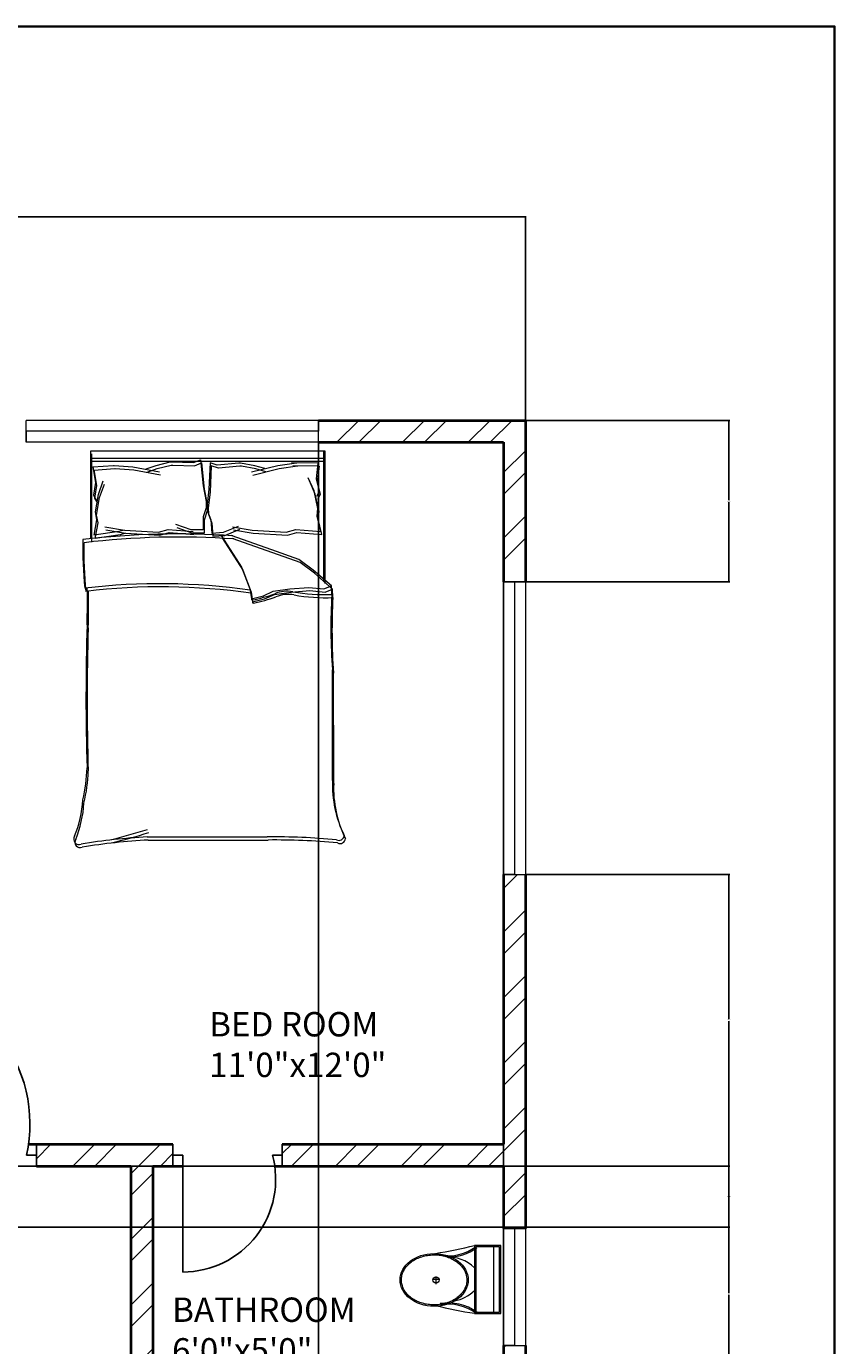
# Model space of a CAD drawing. Units: inches. Extents: x 2063 to 2617, y 1299 to 2210.
# Tile 22 of 22: x 2451 to 2617, y 1939 to 2210. Entities that reach past the tile are written whole.
import ezdxf

# ---------------------------------------------------------------- set-up
doc = ezdxf.new("R2010")
doc.units = ezdxf.units.IN
for name, color, linetype, lineweight in [('A-ANNO-DIMS', 2, 'Continuous', 18), ('A-ANNO-TTLB', 7, 'Continuous', 35), ('A-AREA-IDEN', 7, 'Continuous', 18), ('A-DOOR', 11, 'Continuous', 25), ('A-FLOR-FIXT', 8, 'Continuous', 18), ('A-FURN', 8, 'Continuous', 18), ('A-GLAZ', 123, 'Continuous', 18), ('A-WALL', 7, 'Continuous', 40)]:
    doc.layers.add(name, color=color, linetype=linetype, lineweight=lineweight)
doc.layers.add('A-WALL-PATT', color=215, linetype='Continuous', lineweight=13, true_color=0xa953a0)
doc.styles.get("Standard").update_dxf_attribs({"font": 'arial.ttf'})
doc.dimstyles.get("Standard").update_dxf_attribs({"dimtxt": 0.18, "dimasz": 0.18, "dimexe": 0.18, "dimexo": 0.0625, "dimgap": 0.09, "dimtad": 0, "dimtih": 1, "dimtoh": 1, "dimdec": 4, "dimzin": 0, "dimdsep": 46, "dimtxsty": 'Standard', "dimcen": 0.09, "dimadec": 0, "dimazin": 0, "dimtfac": 1, "dimtdec": 4, "dimtofl": 0, "dimtmove": 0, "dimatfit": 3, "dimfxl": 1, "dimtolj": 1, "dimtzin": 0, "dimarcsym": 0})

# ---------------------------------------------------------------- blocks, each defined once
blk = doc.blocks.new('A$C31115884')
for p, q in [((258, 466), (258, 523)), ((283, 498), (223, 498)), ((0, 200), (0, 0)), ((520, 200), (0, 200)), ((10, 190), (10, 10)), ((510, 190), (10, 190)), ((510, 10), (510, 190)), ((520, 0), (520, 200)), ((510, 54), (0, 54)), ((10, 10), (510, 10)), ((0, 0), (520, 0))]:
    blk.add_line(p, q)
blk.add_circle((256, 496), 23.6)
for centre, radius, start, end in [((2778, -205), 2807, 165.4549, 171.7133), ((-295, 403), 365, 324.2091, 9.3499), ((-295, 403), 375, 324.2091, 9.3499), ((139, 406), 293, 315.8436, 2.6563), ((806, 403), 375, 179.2036, 215.7909), ((806, 403), 365, 170.6501, 215.7909), ((3237, 905), 2807, 188.2867, 194.5451), ((384, 406), 293, 190.2774, 224.1564)]:
    blk.add_arc(centre, radius, start, end)
blk.add_ellipse((256, 510), major_axis=(0, -261), ratio=0.772727)
blk.add_open_spline([(256, 259), (263, 259), (270, 260), (288, 262), (299, 265), (320, 273), (330, 278), (350, 291), (360, 299), (378, 316), (386, 326), (402, 347), (409, 358), (421, 383), (427, 395), (436, 422), (440, 436), (445, 465), (447, 480), (448, 509), (448, 524), (445, 553), (443, 568), (436, 596), (432, 610), (422, 636), (416, 649), (402, 672), (395, 683), (379, 703), (370, 712), (351, 728), (341, 735), (321, 746), (310, 751), (289, 757), (278, 759), (256, 761), (245, 761), (223, 757), (212, 754), (191, 746), (181, 741), (161, 728), (151, 720), (133, 703), (125, 693), (110, 672), (103, 660), (90, 636), (85, 623), (76, 596), (72, 582), (67, 553), (66, 538), (64, 509), (65, 494), (68, 465), (70, 450), (77, 422), (81, 408), (91, 382), (97, 370), (111, 346), (118, 335), (135, 316), (144, 307), (162, 291), (172, 284), (193, 273), (203, 269), (225, 262), (236, 260), (250, 259), (253, 259), (256, 259)], degree=3, knots=[0, 0, 0, 0, 0.110105, 0.110105, 0.285049, 0.285049, 0.459994, 0.459994, 0.634938, 0.634938, 0.809882, 0.809882, 0.984827, 0.984827, 1.159771, 1.159771, 1.334715, 1.334715, 1.50966, 1.50966, 1.684604, 1.684604, 1.859549, 1.859549, 2.034493, 2.034493, 2.209437, 2.209437, 2.384382, 2.384382, 2.559326, 2.559326, 2.73427, 2.73427, 2.909215, 2.909215, 3.084159, 3.084159, 3.259103, 3.259103, 3.434048, 3.434048, 3.608992, 3.608992, 3.783936, 3.783936, 3.958881, 3.958881, 4.133825, 4.133825, 4.30877, 4.30877, 4.483714, 4.483714, 4.658658, 4.658658, 4.833603, 4.833603, 5.008547, 5.008547, 5.183491, 5.183491, 5.358436, 5.358436, 5.53338, 5.53338, 5.708324, 5.708324, 5.883269, 5.883269, 6.058213, 6.058213, 6.233158, 6.233158, 6.283185, 6.283185, 6.283185, 6.283185])
blk = doc.blocks.new('BED-DOUBLE')
for p, q in [((3.48, 63.33), (3.48, 81.44)), ((3.48, 63.33), (3.48, 81.44)), ((3.48, 81.44), (51.49, 81.44)), ((51.27, 81.44), (51.27, 54.83)), ((51.27, 81.44), (51.27, 54.83)), ((51.49, 81.44), (51.49, 80.8)), ((3.48, 79.91), (51.27, 79.91)), ((3.48, 79.91), (51.27, 79.91)), ((3.7, 62.69), (3.7, 80.8)), ((3.7, 62.69), (3.7, 80.8)), ((3.7, 79.27), (51.49, 79.27)), ((3.7, 79.27), (51.49, 79.27)), ((16.88, 78.42), (19.77, 79.14)), ((16.88, 78.42), (19.77, 79.14)), ((17.11, 77.78), (20, 78.5)), ((17.11, 77.78), (20, 78.5)), ((19.77, 79.14), (20.09, 79.14)), ((19.77, 79.14), (20.09, 79.14)), ((20, 78.5), (20.32, 78.5)), ((20, 78.5), (20.32, 78.5)), ((20.09, 79.14), (24.54, 79)), ((20.09, 79.14), (24.54, 79)), ((20.32, 78.5), (24.77, 78.36)), ((20.32, 78.5), (24.77, 78.36)), ((24.54, 79), (25.98, 79.57)), ((24.54, 79), (25.98, 79.57)), ((24.77, 78.36), (26.21, 78.93)), ((24.77, 78.36), (26.21, 78.93)), ((25.98, 79.57), (26.56, 74.22)), ((25.98, 79.57), (26.56, 74.22)), ((26.21, 78.93), (26.79, 73.58)), ((26.21, 78.93), (26.79, 73.58)), ((27.98, 78.95), (27.73, 73.58)), ((27.98, 78.95), (27.73, 73.58)), ((29.46, 78.46), (27.98, 78.95)), ((29.46, 78.46), (27.98, 78.95)), ((33.88, 78.89), (29.46, 78.46)), ((33.88, 78.89), (29.46, 78.46)), ((34.21, 78.91), (33.88, 78.89)), ((34.2, 78.91), (33.88, 78.89)), ((37.14, 78.37), (34.2, 78.91)), ((37.14, 78.37), (34.21, 78.91)), ((45.71, 78.9), (41.91, 78.37)), ((45.71, 78.9), (41.91, 78.37)), ((50.11, 78.89), (44.71, 78.98)), ((44.71, 78.98), (45.71, 78.9)), ((50.11, 78.89), (44.71, 78.98)), ((44.71, 78.98), (45.71, 78.9)), ((50.11, 78.89), (49.73, 75.68)), ((50.11, 78.89), (49.73, 75.68)), ((51.49, 80.8), (51.49, 54.19)), ((51.49, 80.8), (51.49, 54.19)), ((3.89, 78.13), (4.47, 74.95)), ((3.9, 78.11), (8.18, 78.43)), ((3.9, 78.11), (8.18, 78.43)), ((3.9, 78.13), (4.47, 74.95)), ((4.12, 77.49), (4.7, 74.31)), ((4.12, 77.49), (4.7, 74.31)), ((4.13, 77.47), (8.41, 77.8)), ((4.13, 77.47), (8.41, 77.8)), ((8.18, 78.43), (8.29, 78.42)), ((8.18, 78.43), (8.29, 78.42)), ((8.29, 78.42), (12.11, 78.13)), ((8.29, 78.42), (12.11, 78.13)), ((8.41, 77.8), (8.51, 77.78)), ((8.41, 77.8), (8.51, 77.78)), ((8.51, 77.78), (12.34, 77.49)), ((8.51, 77.78), (12.34, 77.49)), ((12.11, 78.13), (17.6, 77.12)), ((12.11, 78.13), (17.6, 77.12)), ((12.34, 77.49), (17.83, 76.48)), ((12.34, 77.49), (17.83, 76.48)), ((14.86, 77.69), (16.88, 78.42)), ((14.86, 77.69), (16.88, 78.42)), ((15.08, 77.05), (17.11, 77.78)), ((15.08, 77.05), (17.11, 77.78)), ((28.21, 78.31), (27.96, 72.94)), ((28.21, 78.31), (27.96, 72.94)), ((29.68, 77.83), (28.21, 78.31)), ((29.68, 77.83), (28.21, 78.31)), ((34.11, 78.25), (29.68, 77.83)), ((34.11, 78.25), (29.68, 77.83)), ((34.43, 78.27), (34.11, 78.25)), ((34.43, 78.27), (34.11, 78.25)), ((37.36, 77.73), (34.43, 78.27)), ((37.36, 77.73), (34.43, 78.27)), ((41.91, 78.37), (36.5, 77.02)), ((41.91, 78.37), (36.5, 77.02)), ((42.14, 77.73), (36.72, 76.38)), ((42.14, 77.73), (36.72, 76.38)), ((39.2, 77.77), (37.14, 78.37)), ((39.2, 77.77), (37.14, 78.37)), ((39.43, 77.13), (37.36, 77.73)), ((39.43, 77.13), (37.36, 77.73)), ((45.94, 78.26), (42.14, 77.73)), ((45.94, 78.26), (42.14, 77.73)), ((50.34, 78.25), (44.94, 78.34)), ((44.94, 78.34), (45.94, 78.26)), ((50.34, 78.25), (44.94, 78.34)), ((44.94, 78.34), (45.94, 78.26)), ((49.31, 73.19), (48.13, 75.87)), ((49.31, 73.19), (48.13, 75.87)), ((50.34, 78.25), (49.96, 75.04)), ((50.34, 78.25), (49.96, 75.04)), ((4.47, 74.95), (4.04, 72.34)), ((4.47, 74.95), (4.04, 72.34)), ((4.7, 74.31), (4.27, 71.7)), ((4.7, 74.31), (4.27, 71.7)), ((5.05, 72.49), (6.06, 75.24)), ((5.05, 72.49), (6.06, 75.24)), ((5.28, 71.85), (6.29, 74.6)), ((5.28, 71.85), (6.29, 74.6)), ((26.56, 74.22), (27.14, 71.04)), ((26.56, 74.22), (27.14, 71.04)), ((26.79, 73.58), (27.37, 70.4)), ((26.79, 73.58), (27.37, 70.4)), ((27.73, 73.58), (27.36, 70.37)), ((27.73, 73.58), (27.36, 70.37)), ((49.54, 72.55), (48.36, 75.23)), ((49.54, 72.55), (48.36, 75.23)), ((50.11, 69.61), (49.31, 73.19)), ((50.11, 69.61), (49.31, 73.19)), ((49.73, 75.68), (50.33, 73.11)), ((49.73, 75.68), (50.33, 73.11)), ((50.33, 73.11), (49.81, 72.06)), ((50.33, 73.11), (49.82, 72.06)), ((49.96, 75.04), (50.56, 72.47)), ((49.96, 75.04), (50.56, 72.47)), ((4.04, 72.34), (4.62, 71.33)), ((4.04, 72.34), (4.62, 71.33)), ((4.27, 71.7), (4.85, 70.69)), ((4.27, 71.7), (4.85, 70.69)), ((4.47, 68.87), (5.05, 72.49)), ((4.47, 68.87), (5.05, 72.49)), ((4.7, 68.23), (5.28, 71.85)), ((4.7, 68.23), (5.28, 71.85)), ((27.14, 71.04), (27.14, 69.74)), ((27.14, 71.04), (27.14, 69.74)), ((27.37, 70.4), (27.37, 69.1)), ((27.37, 70.4), (27.37, 69.1)), ((27.96, 72.94), (27.58, 69.73)), ((27.96, 72.94), (27.58, 69.73)), ((50.34, 68.98), (49.54, 72.55)), ((50.34, 68.98), (49.54, 72.55)), ((50.56, 72.47), (50.04, 71.42)), ((50.56, 72.47), (50.04, 71.42)), ((4.76, 67.28), (4.47, 68.87)), ((4.76, 67.28), (4.47, 68.87)), ((4.99, 66.64), (4.7, 68.23)), ((4.99, 66.64), (4.7, 68.23)), ((27.14, 69.74), (26.56, 67.86)), ((27.14, 69.74), (26.56, 67.86)), ((26.56, 67.86), (26.56, 65.18)), ((26.56, 67.86), (26.56, 65.18)), ((27.37, 69.1), (26.79, 67.22)), ((27.37, 69.1), (26.79, 67.22)), ((27.36, 70.37), (27.44, 69.07)), ((27.36, 70.37), (27.44, 69.07)), ((27.44, 69.07), (28.13, 67.23)), ((27.44, 69.07), (28.13, 67.23)), ((27.58, 69.73), (27.66, 68.43)), ((27.58, 69.73), (27.66, 68.43)), ((27.66, 68.43), (28.36, 66.59)), ((27.66, 68.43), (28.36, 66.59)), ((49.92, 68.01), (50.11, 69.61)), ((49.92, 68.01), (50.11, 69.61)), ((50.7, 64.87), (49.92, 68.01)), ((50.7, 64.87), (49.92, 68.01)), ((50.15, 67.37), (50.34, 68.98)), ((50.15, 67.37), (50.34, 68.98)), ((4.18, 64.1), (4.76, 67.28)), ((4.18, 64.1), (4.76, 67.28)), ((4.41, 63.46), (4.99, 66.64)), ((4.41, 63.46), (4.99, 66.64)), ((6.38, 65.82), (10.41, 65.15)), ((6.38, 65.82), (10.41, 65.15)), ((6.61, 65.18), (10.64, 64.51)), ((6.61, 65.18), (10.64, 64.51)), ((10.41, 65.15), (9.28, 64.83)), ((10.41, 65.15), (9.28, 64.83)), ((10.41, 65.15), (17.42, 64.72)), ((10.41, 65.15), (17.42, 64.72)), ((17.42, 64.72), (19.38, 65.27)), ((17.42, 64.72), (19.38, 65.27)), ((19.38, 65.27), (24.52, 64.87)), ((19.38, 65.27), (24.52, 64.87)), ((24.1, 65.18), (20.96, 66.27)), ((24.1, 65.18), (20.96, 66.27)), ((24.33, 64.54), (21.19, 65.63)), ((24.33, 64.54), (21.19, 65.63)), ((26.56, 65.18), (24.1, 65.18)), ((26.56, 65.18), (24.1, 65.18)), ((26.79, 67.22), (26.79, 64.54)), ((26.79, 67.22), (26.79, 64.54)), ((28.13, 67.23), (28.3, 64.55)), ((28.13, 67.23), (28.3, 64.55)), ((28.36, 66.59), (28.53, 63.91)), ((28.36, 66.59), (28.53, 63.91)), ((30.75, 64.7), (33.82, 65.99)), ((30.75, 64.7), (33.82, 65.99)), ((30.98, 64.06), (34.05, 65.35)), ((30.98, 64.06), (34.05, 65.35)), ((32.56, 65.82), (36.6, 65.15)), ((32.56, 65.82), (36.6, 65.15)), ((32.79, 65.18), (36.83, 64.51)), ((32.79, 65.18), (36.82, 64.51)), ((36.6, 65.15), (43.61, 64.72)), ((36.6, 65.15), (43.61, 64.72)), ((43.61, 64.72), (45.57, 65.27)), ((43.61, 64.72), (45.57, 65.27)), ((45.57, 65.27), (50.7, 64.87)), ((45.57, 65.27), (50.7, 64.87)), ((50.93, 64.23), (50.15, 67.37)), ((50.93, 64.23), (50.15, 67.37)), ((9.28, 64.83), (4.18, 64.1)), ((9.28, 64.83), (4.18, 64.1)), ((9.51, 64.19), (4.41, 63.46)), ((9.51, 64.19), (4.41, 63.46)), ((10.64, 64.51), (9.51, 64.19)), ((10.64, 64.51), (9.51, 64.19)), ((10.64, 64.51), (17.65, 64.08)), ((10.64, 64.51), (17.65, 64.08)), ((17.65, 64.08), (19.61, 64.64)), ((17.65, 64.08), (19.61, 64.64)), ((19.61, 64.64), (24.74, 64.23)), ((19.61, 64.64), (24.74, 64.23)), ((26.79, 64.54), (24.33, 64.54)), ((26.79, 64.54), (24.33, 64.54)), ((28.3, 64.55), (30.75, 64.7)), ((28.3, 64.55), (30.75, 64.7)), ((28.53, 63.91), (30.98, 64.06)), ((28.53, 63.91), (30.98, 64.06)), ((30.26, 64.06), (34.45, 57.57)), ((30.26, 64.06), (34.45, 57.57)), ((30.49, 63.42), (34.68, 56.93)), ((30.49, 63.42), (34.68, 56.93)), ((40.64, 61.13), (32.31, 64.06)), ((40.64, 61.13), (32.31, 64.06)), ((40.87, 60.49), (32.53, 63.42)), ((40.87, 60.49), (32.54, 63.42)), ((36.82, 64.51), (43.83, 64.08)), ((36.83, 64.51), (43.84, 64.08)), ((43.83, 64.08), (45.8, 64.64)), ((43.84, 64.08), (45.8, 64.64)), ((45.8, 64.64), (50.93, 64.23)), ((45.8, 64.64), (50.93, 64.23)), ((46.22, 59.11), (40.64, 61.13)), ((46.22, 59.11), (40.64, 61.13)), ((46.45, 58.48), (40.87, 60.49)), ((46.45, 58.48), (40.87, 60.49)), ((34.45, 57.57), (36.15, 53.08)), ((34.45, 57.57), (36.15, 53.08)), ((34.68, 56.93), (36.38, 52.44)), ((34.68, 56.93), (36.38, 52.44)), ((49.16, 56.95), (46.22, 59.11)), ((49.16, 56.95), (46.22, 59.11)), ((49.39, 56.31), (46.45, 58.48)), ((49.39, 56.31), (46.45, 58.48)), ((52.87, 53.7), (49.16, 56.95)), ((52.87, 53.7), (49.16, 56.95)), ((53.1, 53.06), (49.39, 56.31)), ((53.1, 53.06), (49.39, 56.31)), ((36.15, 53.08), (36.46, 51.07)), ((36.15, 53.08), (36.46, 51.07)), ((36.38, 52.44), (36.69, 50.43)), ((36.38, 52.44), (36.69, 50.43)), ((36.46, 51.07), (38.94, 51.69)), ((36.46, 51.07), (38.94, 51.69)), ((38.94, 51.69), (40.95, 52.61)), ((38.94, 51.69), (40.95, 52.61)), ((39.17, 51.05), (41.18, 51.97)), ((39.17, 51.05), (41.18, 51.97)), ((40.95, 52.61), (44.36, 53.08)), ((40.95, 52.61), (44.36, 53.08)), ((41.18, 51.97), (44.59, 52.44)), ((41.18, 51.97), (44.59, 52.44)), ((44.36, 53.08), (48.23, 53.39)), ((44.36, 53.08), (48.23, 53.39)), ((44.59, 52.44), (48.46, 52.75)), ((44.59, 52.44), (48.46, 52.75)), ((48.23, 53.39), (51.33, 53.08)), ((48.23, 53.39), (51.33, 53.08)), ((48.46, 52.75), (51.56, 52.44)), ((48.46, 52.75), (51.56, 52.44)), ((51.33, 53.08), (52.87, 53.7)), ((51.33, 53.08), (52.87, 53.7)), ((51.56, 52.44), (53.1, 53.06)), ((51.56, 52.44), (53.1, 53.06)), ((52.95, 51.95), (52.87, 53.7, 3.87)), ((52.95, 51.95), (52.87, 53.7, 3.87)), ((53.18, 51.31), (53.1, 53.06, 3.87)), ((53.18, 51.31), (53.1, 53.06, 3.87)), ((36.69, 50.43), (39.17, 51.05)), ((36.69, 50.43), (39.17, 51.05)), ((15.06, 2.2), (39.68, 2.2)), ((15.06, 2.2), (39.68, 2.2)), ((15.29, 1.56), (39.91, 1.56)), ((15.29, 1.56), (39.91, 1.56))]:
    blk.add_line(p, q)
for centre, radius, start, end in [((85.16, 61.35), 83.31, 178.7218, 185.604), ((85.16, 61.35), 83.31, 178.7218, 185.604), ((21.36, -100.61), 164.97, 86.0865, 96.7821), ((21.36, -100.61), 164.97, 86.0865, 96.7821), ((85.39, 60.71), 83.31, 178.7218, 185.604), ((85.39, 60.71), 83.31, 178.7218, 185.604), ((21.59, -101.25), 164.97, 86.0865, 96.7821), ((21.59, -101.25), 164.97, 86.0865, 96.7821), ((17.76, -74.87), 129.02, 81.7845, 96.9006), ((17.76, -74.87), 129.02, 81.7845, 96.9006), ((17.98, -75.51), 129.02, 81.7845, 96.9006), ((17.98, -75.51), 129.02, 81.7845, 96.9006), ((-167.31, 50.27), 170.11, 358.4762, 1.0082), ((-167.31, 50.27), 170.11, 358.4762, 1.0082), ((-167.08, 49.63), 170.11, 358.4762, 1.0082), ((-167.08, 49.63), 170.11, 358.4762, 1.0082), ((31.15, 79.96), 29.65, 280.6617, 289.8806), ((31.15, 79.96), 29.65, 280.6617, 289.8806), ((31.38, 79.32), 29.65, 280.6617, 289.8806), ((31.38, 79.32), 29.65, 280.6617, 289.8806), ((43.74, 46.38), 6.22, 78.6608, 113.7384), ((43.74, 46.38), 6.22, 78.6608, 113.7384), ((43.97, 45.74), 6.22, 78.6608, 113.7384), ((43.97, 45.74), 6.22, 78.6608, 113.7384), ((51.33, 88.1), 36.18, 259.8763, 272.5657), ((51.33, 88.1), 36.18, 259.8763, 272.5657), ((51.56, 87.46), 36.18, 259.8763, 272.5657), ((51.56, 87.46), 36.18, 259.8763, 272.5657), ((182.27, 45.13), 129.5, 176.9791, 183.8365), ((182.27, 45.13), 129.5, 176.9791, 183.8365), ((36.64, 51), 0.185, 160.2464, 271.1377), ((36.64, 51), 0.185, 160.2464, 271.1377), ((36.87, 50.36), 0.185, 160.2464, 271.1377), ((36.86, 50.36), 0.185, 160.2464, 271.1377), ((182.49, 44.49), 129.5, 176.9791, 183.8365), ((182.49, 44.49), 129.5, 176.9791, 183.8365), ((484.82, 30.83), 482.31, 178.2277, 181.7185), ((484.82, 30.83), 482.31, 178.2277, 181.7185), ((485.05, 30.19), 482.31, 178.2277, 181.7185), ((485.05, 30.19), 482.31, 178.2277, 181.7185), ((-4508.74, 13.62), 4561.86, 0.00217, 0.28689), ((-4508.74, 13.62), 4561.86, 0.00217, 0.28689), ((-4508.51, 12.98), 4561.86, 0.00217, 0.28689), ((-4508.51, 12.98), 4561.86, 0.00217, 0.28689), ((-26.9, 16.93), 29.63, 346.0648, 358.9113), ((-26.9, 16.93), 29.63, 346.0648, 358.9113), ((-26.67, 16.29), 29.63, 346.0648, 358.9113), ((-26.67, 16.29), 29.63, 346.0648, 358.9113), ((76.16, 12.78), 23.07, 177.4714, 206.4681), ((76.16, 12.78), 23.07, 177.4714, 206.4681), ((76.39, 12.14), 23.07, 177.4714, 206.4681), ((76.39, 12.14), 23.07, 177.4714, 206.4681), ((-21.66, 11.17), 23.56, 337.9751, 356.652), ((-21.66, 11.17), 23.56, 337.9751, 356.652), ((-21.43, 10.53), 23.56, 337.9751, 356.652), ((-21.43, 10.53), 23.56, 337.9751, 356.652), ((-17.22, 105.16), 106.46, 283.3832, 287.7053), ((-17.22, 105.16), 106.46, 283.3832, 287.7053), ((-16.99, 104.52), 106.46, 283.3832, 287.7053), ((-16.99, 104.52), 106.46, 283.3832, 287.7053), ((1.09, 1.73), 1.09, 146.1736, 293.4781), ((1.09, 1.73), 1.09, 146.1736, 293.4781), ((1.32, 1.09), 1.09, 146.1736, 293.4781), ((1.32, 1.09), 1.09, 146.1736, 293.4781), ((21.43, -119.39), 121.76, 92.9958, 99.4091), ((21.43, -119.39), 121.76, 92.9958, 99.4091), ((21.66, -120.03), 121.76, 92.9958, 99.4091), ((21.66, -120.03), 121.76, 92.9958, 99.4091), ((41.15, -130.83), 133.04, 84.4998, 90.6351), ((41.15, -130.83), 133.04, 84.4998, 90.6351), ((41.38, -131.47), 133.04, 84.4998, 90.6351), ((41.38, -131.47), 133.04, 84.4998, 90.6351), ((54.41, 2.57), 1.1, 242.6588, 356.02), ((54.41, 2.57), 1.1, 242.6588, 356.02), ((54.64, 1.93), 1.1, 242.6588, 356.02), ((54.64, 1.93), 1.1, 242.6588, 356.02)]:
    blk.add_arc(centre, radius, start, end)
blk = doc.blocks.new('WIN-60IN')
for p, q in [((0, 60), (4.5, 60)), ((0, 60), (0, 0)), ((4.5, 60), (2.25, 60)), ((2.25, 60), (2.25, 0)), ((4.5, 60), (4.5, 0)), ((2.25, 0), (0, 0)), ((0, 0), (4.5, 0))]:
    blk.add_line(p, q)
blk = doc.blocks.new('WIN-24IN')
for p, q in [((0, 24), (4.5, 24)), ((0, 24), (0, 0)), ((4.5, 24), (2.25, 24)), ((2.25, 24), (2.25, 0)), ((4.5, 24), (4.5, 0)), ((2.25, 0), (0, 0)), ((0, 0), (4.5, 0))]:
    blk.add_line(p, q)
blk = doc.blocks.new('*D31')
at = {"layer": 'A-ANNO-DIMS', "color": 0, "lineweight": -2, "transparency": 16777216}
for p, q in [((2123.14, 2128.87), (2123.14, 2170.74)), ((2123.32, 2170.56), (2338, 2170.56)), ((2553.46, 2170.56), (2338.79, 2170.56)), ((2553.64, 2128.87), (2553.64, 2170.74))]:
    blk.add_line(p, q, dxfattribs=at)
at = {"layer": 'A-ANNO-DIMS', "color": 0, "transparency": 16777216}
for points in [[(2123.32, 2170.59), (2123.32, 2170.53), (2123.14, 2170.56)], [(2553.46, 2170.59), (2553.46, 2170.53), (2553.64, 2170.56)]]:
    blk.add_solid(points, dxfattribs=at)
at = {"layer": 'Defpoints', "color": 0, "transparency": 16777216}
for p in [(2553.64, 2170.56), (2123.14, 2128.81), (2553.64, 2128.81)]:
    blk.add_point(p, dxfattribs=at)
at = {"layer": 'A-ANNO-DIMS', "color": 0, "transparency": 16777216, "insert": (2338.39, 2170.56), "char_height": 0.18, "attachment_point": 5}
blk.add_mtext('\\A1;430.5', dxfattribs=at)
blk = doc.blocks.new('*D46')
at = {"layer": 'A-ANNO-DIMS', "color": 0, "lineweight": -2, "transparency": 16777216}
for p, q in [((2549.21, 1975.81), (2595.57, 1975.81)), ((2595.39, 1975.63), (2595.39, 1949.74)), ((2595.39, 1923.49), (2595.39, 1949.38)), ((2549.21, 1923.31), (2595.57, 1923.31))]:
    blk.add_line(p, q, dxfattribs=at)
at = {"layer": 'A-ANNO-DIMS', "color": 0, "transparency": 16777216}
for points in [[(2595.36, 1975.63), (2595.42, 1975.63), (2595.39, 1975.81)], [(2595.36, 1923.49), (2595.42, 1923.49), (2595.39, 1923.31)]]:
    blk.add_solid(points, dxfattribs=at)
at = {"layer": 'Defpoints', "color": 0, "transparency": 16777216}
for p in [(2549.14, 1975.81), (2595.39, 1975.81), (2549.14, 1923.31)]:
    blk.add_point(p, dxfattribs=at)
at = {"layer": 'A-ANNO-DIMS', "color": 0, "transparency": 16777216, "insert": (2595.39, 1949.56), "char_height": 0.18, "attachment_point": 5}
blk.add_mtext('\\A1;52.5', dxfattribs=at)
blk = doc.blocks.new('*D47')
at = {"layer": 'A-ANNO-DIMS', "color": 0, "lineweight": -2, "transparency": 16777216}
for p, q in [((2553.71, 2035.66), (2595.57, 2035.66)), ((2595.39, 2035.48), (2595.39, 2005.92)), ((2595.39, 1975.99), (2595.39, 2005.56)), ((2549.21, 1975.81), (2595.57, 1975.81))]:
    blk.add_line(p, q, dxfattribs=at)
at = {"layer": 'A-ANNO-DIMS', "color": 0, "transparency": 16777216}
for points in [[(2595.36, 2035.48), (2595.42, 2035.48), (2595.39, 2035.66)], [(2595.36, 1975.99), (2595.42, 1975.99), (2595.39, 1975.81)]]:
    blk.add_solid(points, dxfattribs=at)
at = {"layer": 'Defpoints', "color": 0, "transparency": 16777216}
for p in [(2553.64, 2035.66), (2595.39, 2035.66), (2549.14, 1975.81)]:
    blk.add_point(p, dxfattribs=at)
at = {"layer": 'A-ANNO-DIMS', "color": 0, "transparency": 16777216, "insert": (2595.39, 2005.74), "char_height": 0.18, "attachment_point": 5}
blk.add_mtext('\\A1;59.85', dxfattribs=at)
blk = doc.blocks.new('*D48')
at = {"layer": 'A-ANNO-DIMS', "color": 0, "lineweight": -2, "transparency": 16777216}
for p, q in [((2553.71, 2128.81), (2595.57, 2128.81)), ((2595.39, 2128.63), (2595.39, 2112.42)), ((2595.39, 2095.84), (2595.39, 2112.06)), ((2549.21, 2095.66), (2595.57, 2095.66))]:
    blk.add_line(p, q, dxfattribs=at)
at = {"layer": 'A-ANNO-DIMS', "color": 0, "transparency": 16777216}
for points in [[(2595.36, 2128.63), (2595.42, 2128.63), (2595.39, 2128.81)], [(2595.36, 2095.84), (2595.42, 2095.84), (2595.39, 2095.66)]]:
    blk.add_solid(points, dxfattribs=at)
at = {"layer": 'Defpoints', "color": 0, "transparency": 16777216}
for p in [(2553.64, 2128.81), (2595.39, 2128.81), (2549.14, 2095.66)]:
    blk.add_point(p, dxfattribs=at)
at = {"layer": 'A-ANNO-DIMS', "color": 0, "transparency": 16777216, "insert": (2595.39, 2112.24), "char_height": 0.18, "attachment_point": 5}
blk.add_mtext('\\A1;33.15', dxfattribs=at)
blk = doc.blocks.new('*D52')
at = {"layer": 'A-ANNO-DIMS', "color": 0, "lineweight": -2, "transparency": 16777216}
for p, q in [((2511.17, 2124.25), (2511.17, 1317.7)), ((2549.14, 2124.25), (2549.14, 1317.7)), ((2511.35, 1317.88), (2529.69, 1317.88)), ((2548.96, 1317.88), (2530.62, 1317.88))]:
    blk.add_line(p, q, dxfattribs=at)
at = {"layer": 'A-ANNO-DIMS', "color": 0, "transparency": 16777216}
for points in [[(2511.35, 1317.91), (2511.35, 1317.85), (2511.17, 1317.88)], [(2548.96, 1317.91), (2548.96, 1317.85), (2549.14, 1317.88)]]:
    blk.add_solid(points, dxfattribs=at)
at = {"layer": 'Defpoints', "color": 0, "transparency": 16777216}
for p in [(2511.17, 2124.31), (2549.14, 2124.31), (2549.14, 1317.88)]:
    blk.add_point(p, dxfattribs=at)
at = {"layer": 'A-ANNO-DIMS', "color": 0, "transparency": 16777216, "insert": (2530.16, 1317.88), "char_height": 0.18, "attachment_point": 5}
blk.add_mtext('\\A1;37.974', dxfattribs=at)
blk = doc.blocks.new('*D67')
at = {"layer": 'A-ANNO-DIMS', "color": 0, "lineweight": -2, "transparency": 16777216}
for p, q in [((2127.71, 1975.81), (2595.57, 1975.81)), ((2595.39, 1975.63), (2595.39, 1969.73)), ((2595.39, 1963.46), (2595.39, 1969.36)), ((2128.42, 1963.28), (2595.57, 1963.28))]:
    blk.add_line(p, q, dxfattribs=at)
at = {"layer": 'A-ANNO-DIMS', "color": 0, "transparency": 16777216}
for points in [[(2595.36, 1975.63), (2595.42, 1975.63), (2595.39, 1975.81)], [(2595.36, 1963.46), (2595.42, 1963.46), (2595.39, 1963.28)]]:
    blk.add_solid(points, dxfattribs=at)
at = {"layer": 'Defpoints', "color": 0, "transparency": 16777216}
for p in [(2127.64, 1975.81), (2128.36, 1963.28), (2595.39, 1963.28)]:
    blk.add_point(p, dxfattribs=at)
at = {"layer": 'A-ANNO-DIMS', "color": 0, "transparency": 16777216, "insert": (2595.39, 1969.55), "char_height": 0.18, "attachment_point": 5}
blk.add_mtext('\\A1;12.533', dxfattribs=at)

msp = doc.modelspace()

# ---------------------------------------------------------------- hatches: boundary and pattern name
at = {"layer": 'A-WALL-PATT'}
h = msp.add_hatch(dxfattribs=at)
h.set_pattern_fill('ANSI32', color=256)
h.paths.add_polyline_path([(2553.6442, 2128.8122), (2511.1703, 2128.8122), (2511.1703, 2124.3122), (2549.1442, 2124.3122), (2549.1442, 2095.662), (2553.6442, 2095.662)])
h.paths.add_polyline_path([(2553.6442, 2035.662), (2549.1442, 2035.662), (2549.1442, 1980.3122), (2503.7214, 1980.3122), (2503.7214, 1975.8122), (2549.1442, 1975.8122), (2549.1442, 1962.9693), (2553.6442, 1962.9693)])
h.paths.add_polyline_path([(2553.6442, 1938.9693), (2549.1442, 1938.9693), (2549.1442, 1927.8122), (2477.1442, 1927.8122), (2477.1442, 1975.8122), (2481.2918, 1975.8122), (2481.2918, 1980.3122), (2453.2648, 1980.3122), (2453.2648, 1975.8122), (2472.6442, 1975.8122), (2472.6442, 1868.3122), (2400.6442, 1868.3122), (2400.6442, 1861.3782), (2405.1442, 1861.3782), (2405.1442, 1863.8122), (2480.9699, 1863.8122), (2480.9699, 1866.0622), (2480.9699, 1868.3122), (2477.1442, 1868.3122), (2477.1442, 1923.3122), (2549.1442, 1923.3122), (2549.1442, 1908.8504), (2553.6442, 1908.8504)])
h.paths.add_polyline_path([(2553.6442, 1884.8504), (2549.1442, 1884.8504), (2549.1442, 1868.3122), (2501.0636, 1868.3122), (2501.0636, 1863.8122), (2549.1442, 1863.8122), (2549.1442, 1826.0298), (2553.6442, 1826.0298)])
h.paths.add_polyline_path([(2388.1504, 1980.3122), (2340.6442, 1980.3122), (2340.6442, 2124.3122), (2358.7501, 2124.3122), (2358.7501, 2128.8122), (2316.3482, 2128.8122), (2316.3482, 2124.3122), (2336.1442, 2124.3122), (2336.1442, 1980.3122), (2289.1737, 1980.3122), (2289.1737, 1975.8122), (2336.1442, 1975.8122), (2336.1442, 1619.3122), (2333.1433, 1619.3122), (2333.1433, 1614.8122), (2344.1671, 1614.8122), (2344.1671, 1617.0622), (2344.1671, 1619.3122), (2340.6442, 1619.3122), (2340.6442, 1975.8122), (2388.1504, 1975.8122), (2388.1504, 1978.0622)])
h.paths.add_polyline_path([(2290.1442, 1614.8122), (2301.4594, 1614.8122), (2301.4594, 1617.0622), (2301.4594, 1619.3122), (2285.6442, 1619.3122), (2285.6442, 1566.8122), (2280.8619, 1566.8122), (2280.8619, 1564.5622), (2280.8619, 1562.3122), (2285.6442, 1562.3122), (2285.6442, 1442.3122), (2281.7879, 1442.3122), (2281.7879, 1437.8122), (2285.6442, 1437.8122), (2285.6442, 1401.8122), (2290.1442, 1401.8122)])
h.paths.add_polyline_path([(2549.1442, 1731.8122), (2405.1442, 1731.8122), (2405.1442, 1834.4638), (2402.8942, 1834.4638), (2400.6442, 1834.4638), (2400.6442, 1727.3122), (2549.1442, 1727.3122)])
h.paths.add_polyline_path([(2553.6442, 1766.0298), (2551.3942, 1766.0298), (2549.1442, 1766.0298), (2549.1442, 1686.7767), (2553.6442, 1686.7767)])
h.paths.add_polyline_path([(2553.6442, 1638.7767), (2551.3942, 1638.7767), (2549.1442, 1638.7767), (2549.1442, 1619.3122), (2448.6442, 1619.3122), (2448.6442, 1610.5671), (2450.8942, 1610.5671), (2453.1442, 1610.5671), (2453.1442, 1614.8122), (2549.1442, 1614.8122), (2549.1442, 1601.6421), (2553.6442, 1601.6421)])
h.paths.add_polyline_path([(2553.6442, 1577.6421), (2551.3942, 1577.6421), (2549.1442, 1577.6421), (2549.1442, 1566.8122), (2453.1442, 1566.8122), (2453.1442, 1591.5045), (2451.0335, 1591.5045), (2448.6442, 1591.5045), (2448.6442, 1566.8122), (2434.0475, 1566.8122), (2434.0475, 1562.3122), (2549.1442, 1562.3122), (2549.1442, 1533.48), (2553.6442, 1533.48)])
h.paths.add_polyline_path([(2553.6442, 1473.48), (2549.1442, 1473.48), (2549.1442, 1442.3122), (2502.6258, 1442.3122), (2502.6258, 1437.8122), (2549.1442, 1437.8122), (2549.1442, 1401.8122), (2553.6442, 1401.8122)])
h.paths.add_polyline_path([(2395.6442, 1562.3122), (2400.0901, 1562.3122), (2400.0901, 1564.5622), (2400.0901, 1566.8122), (2395.6442, 1566.8122), (2395.6442, 1619.3122), (2379.1127, 1619.3122), (2379.1127, 1614.8122), (2391.1442, 1614.8122), (2391.1442, 1401.8122), (2395.6442, 1401.8122), (2395.6442, 1437.8122), (2399.2425, 1437.8122), (2399.2425, 1440.0622), (2399.2425, 1442.3122), (2395.6442, 1442.3122)])
h.paths.add_polyline_path([(2442.6258, 1442.3122), (2419.6262, 1442.3122), (2419.6262, 1437.8122), (2442.6258, 1437.8122), (2442.6258, 1440.0622)])
h.paths.add_polyline_path([(2127.6442, 1480.2532), (2125.3942, 1480.2532), (2123.1442, 1480.2532), (2123.1442, 1401.8122), (2127.6442, 1401.8122), (2127.6442, 1437.8122), (2145.1538, 1437.8122), (2145.1538, 1440.0622), (2145.1538, 1442.3122), (2127.6442, 1442.3122)])
h.paths.add_polyline_path([(2259.809, 1442.3122), (2205.1538, 1442.3122), (2205.1538, 1437.8122), (2259.809, 1437.8122), (2259.809, 1440.0622)])
h.paths.add_polyline_path([(2127.6442, 1659.7652), (2123.1442, 1659.7652), (2123.1442, 1605.5161), (2125.3942, 1605.5161), (2127.6442, 1605.5161), (2127.6442, 1614.8122), (2223.6442, 1614.8122), (2223.6442, 1611.2723), (2228.1442, 1611.2723), (2228.1442, 1619.3122), (2127.6442, 1619.3122)])
h.paths.add_polyline_path([(2244.8673, 1566.8122), (2228.1442, 1566.8122), (2228.1442, 1590.8122), (2225.8942, 1590.8122), (2223.6442, 1590.8122), (2223.6442, 1566.8122), (2127.6442, 1566.8122), (2127.6442, 1581.5161), (2123.1442, 1581.5161), (2123.1442, 1540.2532), (2127.6442, 1540.2532), (2127.6442, 1562.3122), (2244.8673, 1562.3122), (2244.8673, 1564.5622)])
h.paths.add_polyline_path([(2172.5174, 1868.3122), (2127.6442, 1868.3122), (2127.6442, 1886.5833), (2123.1442, 1886.5833), (2123.1442, 1832.6633), (2127.6442, 1832.6633), (2127.6442, 1863.8122), (2172.5174, 1863.8122), (2172.5174, 1866.0622)])
h.paths.add_polyline_path([(2276.1442, 1868.3122), (2204.1442, 1868.3122), (2204.1442, 1923.3122), (2204.1442, 1975.8122), (2224.8362, 1975.8122), (2224.8362, 1978.1097), (2224.8362, 1980.3122), (2195.0729, 1980.3122), (2195.0729, 1978.0622), (2195.0729, 1975.8122), (2199.6442, 1975.8122), (2199.6442, 1927.8122), (2127.6442, 1927.8122), (2127.6442, 1942.3492), (2123.1442, 1942.3492), (2123.1442, 1910.5833), (2127.6442, 1910.5833), (2127.6442, 1923.3122), (2199.6442, 1923.3122), (2199.6442, 1868.3122), (2194.8228, 1868.3122), (2194.8228, 1864.7337), (2194.8228, 1863.8122), (2271.6442, 1863.8122), (2271.6442, 1860.0507), (2276.1442, 1860.0507)])
h.paths.add_polyline_path([(2276.1442, 1829.994), (2273.8942, 1829.994), (2271.6442, 1829.994), (2271.6442, 1731.8122), (2127.6442, 1731.8122), (2127.6442, 1772.6633), (2123.1442, 1772.6633), (2123.1442, 1707.7652), (2127.6442, 1707.7652), (2127.6442, 1727.3122), (2276.1442, 1727.3122)])
h.paths.add_polyline_path([(2127.6442, 2022.1152), (2123.1442, 2022.1152), (2123.1442, 1966.3492), (2127.6442, 1966.3492), (2127.6442, 1975.8122), (2174.2082, 1975.8122), (2174.2082, 1978.0622), (2174.2082, 1980.3122), (2127.6442, 1980.3122)])
h.paths.add_polyline_path([(2361.9755, 1678.588), (2398.4558, 1678.588), (2398.4558, 1697.2453), (2361.9755, 1697.2453)], flags=9)
h.paths.add_polyline_path([(2351.5397, 1780.4072), (2386.1987, 1780.4072), (2386.1987, 1790.7107), (2351.5397, 1790.7107)], flags=25)
h.paths.add_polyline_path([(2350.6753, 1940.9321), (2387.6024, 1940.9321), (2387.6024, 1959.5894), (2350.6753, 1959.5894)], flags=25)
h.paths.add_polyline_path([(2254.9545, 1684.638), (2295.0943, 1684.638), (2295.0943, 1703.2953), (2254.9545, 1703.2953)], flags=9)
h.paths.add_polyline_path([(2282.4946, 1782.4438), (2317.1535, 1782.4438), (2317.1535, 1792.7474), (2282.4946, 1792.7474)], flags=9)
h.paths.add_polyline_path([(2270.327, 1939.2854), (2307.254, 1939.2854), (2307.254, 1957.9428), (2270.327, 1957.9428)], flags=9)

# ---------------------------------------------------------------- linework, layer by layer
at = {"layer": 'A-ANNO-TTLB'}
msp.add_lwpolyline([(2062.5792, 2209.6485), (2617.0648, 2209.6485), (2617.0648, 1299.1125), (2062.5792, 1299.1125)], close=True, dxfattribs=at)
at = {"layer": 'A-DOOR'}
for p, q in [((2453.2648, 1980.3122), (2453.2648, 1975.8122)), ((2481.2918, 1975.8122), (2481.2918, 1980.3122)), ((2481.2918, 1980.3122), (2481.2918, 1978.0622)), ((2503.7214, 1980.3122), (2503.7214, 1975.8122)), ((2453.2648, 1978.0622), (2451.2648, 1978.0622)), ((2453.2648, 1975.8122), (2453.2648, 1978.0622)), ((2481.2918, 1978.0622), (2483.2918, 1978.0622)), ((2483.2918, 1978.0622), (2483.2918, 1954.0622)), ((2503.7214, 1978.0622), (2501.7214, 1978.0622)), ((2503.7214, 1975.8122), (2503.7214, 1978.0622))]:
    msp.add_line(p, q, dxfattribs=at)
for centre, radius, start, end in [((2422.2747, 1984.3896), 29.6726, 347.687693, 90), ((2483.2918, 1973.1382), 19.0761, 270, 14.958642)]:
    msp.add_arc(centre, radius, start, end, dxfattribs=at)
at = {"layer": 'A-GLAZ'}
for p, q in [((2549.1442, 2095.662), (2553.6442, 2095.662)), ((2549.1442, 2095.662), (2549.1442, 2035.662)), ((2553.6442, 2095.662), (2551.3942, 2095.662)), ((2551.3942, 2095.662), (2551.3942, 2071.662)), ((2553.6442, 2095.662), (2553.6442, 2035.662)), ((2551.3942, 2071.662), (2551.3942, 2035.662)), ((2551.3942, 2035.662), (2549.1442, 2035.662)), ((2549.1442, 2035.662), (2553.6442, 2035.662))]:
    msp.add_line(p, q, dxfattribs=at)
at = {"layer": 'A-WALL'}
for p, q in [((2511.1703, 2128.8122), (2553.6442, 2128.8122)), ((2511.1703, 2128.8122), (2553.6442, 2128.8122)), ((2553.6442, 2128.8122), (2553.6442, 2095.662)), ((2511.1703, 2124.3122), (2549.1442, 2124.3122)), ((2549.1442, 2124.3122), (2549.1442, 2095.662)), ((2549.1442, 2035.662), (2549.1442, 1980.3122)), ((2553.6442, 2035.662), (2553.6442, 1962.9693)), ((2451.6658, 1980.3122), (2481.2918, 1980.3122)), ((2503.7214, 1980.3122), (2549.1442, 1980.3122)), ((2453.2648, 1975.8122), (2472.6442, 1975.8122)), ((2472.6442, 1975.8122), (2472.6442, 1868.3122)), ((2477.1442, 1975.8122), (2477.1442, 1927.8122)), ((2477.1442, 1975.8122), (2483.2918, 1975.8122)), ((2502.1795, 1975.8122), (2549.1442, 1975.8122)), ((2549.1442, 1975.8122), (2549.1442, 1962.9693)), ((2549.1442, 1938.9693), (2549.1442, 1927.8122)), ((2553.6442, 1938.9693), (2553.6442, 1908.8504))]:
    msp.add_line(p, q, dxfattribs=at)

# ---------------------------------------------------------------- block references
at = {"layer": 'A-FLOR-FIXT', "xscale": 0.0268011493576733, "yscale": 0.0268011493576733, "zscale": 0.0268011493576733, "rotation": 89.99999999999999}
msp.add_blockref('A$C31115884', (2548.55, 1945.5876), dxfattribs=at)
at = {"layer": 'A-FURN'}
msp.add_blockref('BED-DOUBLE', (2460.9378, 2041.145), dxfattribs=at)
at = {"layer": 'A-GLAZ', "extrusion": (0, 0, -1), "zscale": -1, "rotation": 90}
msp.add_blockref('WIN-60IN', (-2451.1701, 2124.3119), dxfattribs=at)
at = {"layer": 'A-GLAZ'}
msp.add_blockref('WIN-24IN', (2549.144, 1938.969), dxfattribs=at)

# ---------------------------------------------------------------- texts
at = {"layer": 'A-AREA-IDEN', "char_height": 5, "attachment_point": 1}
for s, width, insert in [('BED ROOM\\P11\'0"x12\'0"', 206.44031, (2488.7197, 2007.4073)), ('BATHROOM\\P6\'0"x5\'0"', 102.054079, (2481.1209, 1948.8348))]:
    msp.add_mtext_dynamic_manual_height_columns(s, width=width, gutter_width=12.5, heights=[0], dxfattribs=dict(at, insert=insert))

# ---------------------------------------------------------------- dimensions: what is measured, and where the dimension line sits
at = {"layer": 'A-ANNO-DIMS'}
for base, p1, p2, override, picture, middle in [((2553.6442, 2170.5622), (2123.1442, 2128.8122), (2553.6442, 2128.8122), {"dimdec": 1, "dimlfac": 1, "dimrnd": 0, "dimzin": 0, "dimdsep": 46, "dimlunit": 2}, '*D31', (2338.3942, 2170.5622)), ((2549.1442, 1317.8821), (2511.1703, 2124.3122), (2549.1442, 2124.3122), {"dimdec": 3, "dimlfac": 1, "dimrnd": 0, "dimzin": 0, "dimdsep": 46, "dimlunit": 2}, '*D52', (2530.1573, 1317.8821))]:
    dim = msp.add_linear_dim(base=base, p1=p1, p2=p2, dimstyle='Standard', override=override, dxfattribs=at)
    dim.commit()
    dim.dimension.update_dxf_attribs({"geometry": picture, "text_midpoint": middle})
for base, p1, p2, override, picture, middle in [((2595.3943, 2128.8122), (2549.1442, 2095.662), (2553.6442, 2128.8122), {"dimdec": 2, "dimlfac": 1, "dimrnd": 0, "dimzin": 0, "dimdsep": 46, "dimlunit": 2}, '*D48', (2595.3943, 2112.2371)), ((2595.3943, 2035.662), (2549.1442, 1975.8122), (2553.6442, 2035.662), {"dimdec": 2, "dimlfac": 1, "dimrnd": 0, "dimzin": 0, "dimdsep": 46, "dimlunit": 2}, '*D47', (2595.3943, 2005.7371)), ((2595.3943, 1963.2791), (2127.6442, 1975.8122), (2128.3589, 1963.2791), {"dimdec": 3, "dimlfac": 1, "dimrnd": 0, "dimzin": 0, "dimdsep": 46, "dimlunit": 2}, '*D67', (2595.3943, 1969.5457)), ((2595.3943, 1975.8122), (2549.1442, 1923.3122), (2549.1442, 1975.8122), {"dimdec": 1, "dimlfac": 1, "dimrnd": 0, "dimzin": 0, "dimdsep": 46, "dimlunit": 2}, '*D46', (2595.3943, 1949.5622))]:
    dim = msp.add_linear_dim(base=base, p1=p1, p2=p2, angle=90, dimstyle='Standard', override=override, dxfattribs=at)
    dim.commit()
    dim.dimension.update_dxf_attribs({"geometry": picture, "text_midpoint": middle})

doc.saveas('drawing.dxf')
